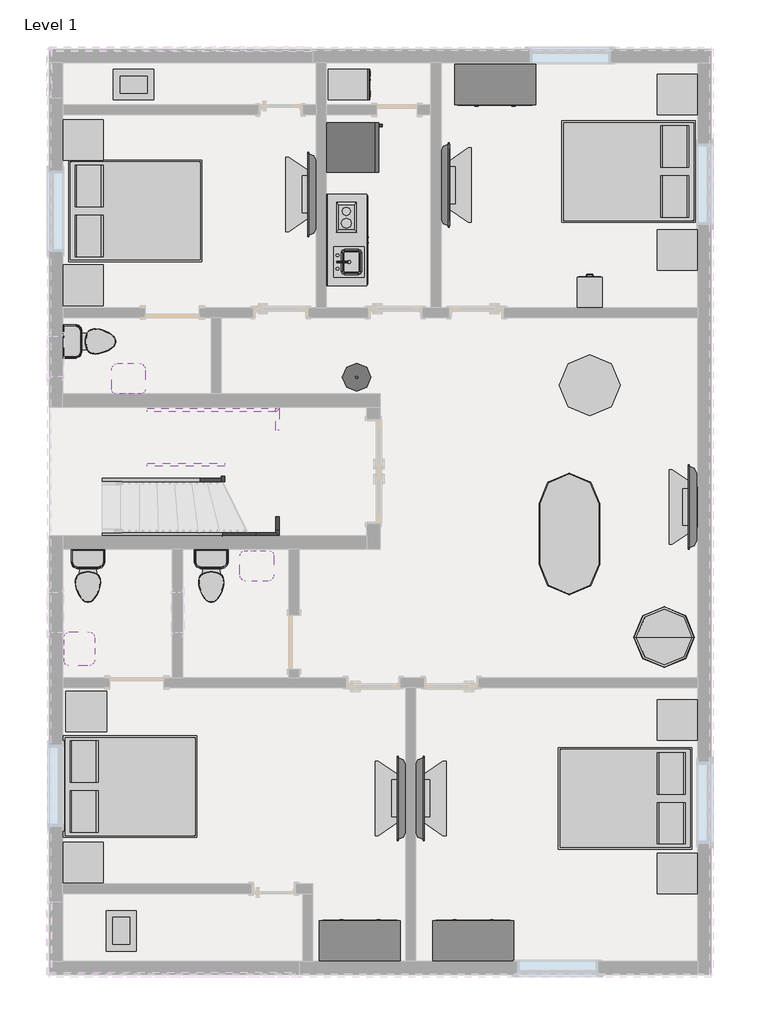
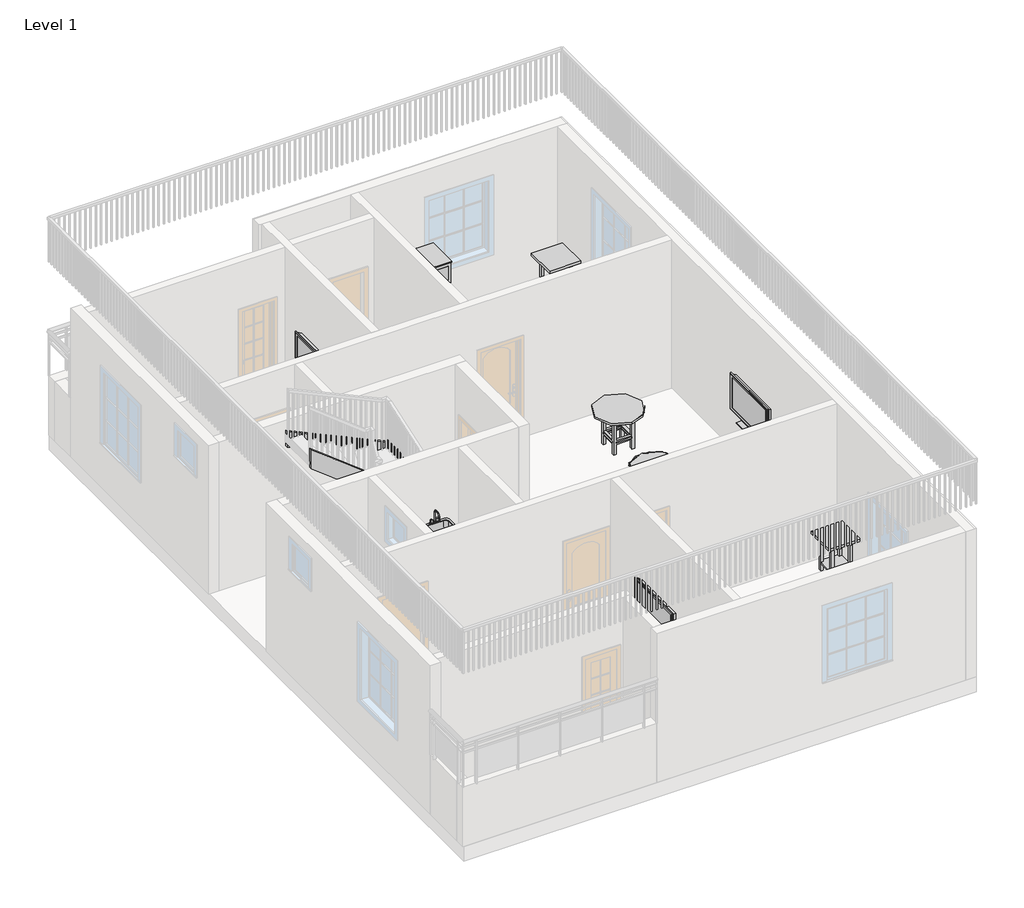
# One storey, part 7 of 7: 32 furniture elements, 10 members, 8 flow terminals, 4 proxies.
"""IFC4 building model written with IfcOpenShell, lengths in millimetres."""

from ifc_helpers import new_model, si_unit, frame, origin, place, context, project, spatial, polyline, outline, extrude, transform, mapped, element, save
from components import proxy_fe84b772, proxy_434a9211, proxy_844211aa, proxy_a13a33b2, flow_terminal_871c2e40, flow_terminal_d49f872f, flow_terminal_62a433f7, toilet_domestic_3d_toilet_domestic_3d_f7549cf7, toilet_domestic_3d_toilet_domestic_3d_183bbd19, furniture_1d2926bd, furniture_552c1472, furniture_95afb093, furniture_2babcf72, furniture_9fa109b2, furniture_fdf74506, tv_stand_tv_stand_6ce107e5, furniture_7122704d, furniture_2c34a4f9, furniture_905aceb5, furniture_5bc9ed15, furniture_c80d6d9c

model = new_model("IFC4")

# Units and contexts
model_context = context("Model", 3, world=origin())
ifc_project = project(units=[si_unit("LENGTHUNIT", "METRE", prefix="MILLI")], contexts=[model_context])

# Site, building, storey
site = spatial("IfcSite", under=ifc_project)
building = spatial("IfcBuilding", under=site)
storey = spatial("IfcBuildingStorey", under=building, Name="Level 1", Elevation=0.0)

# Proxies
placement = place(None, origin())
proxy_shape = proxy_fe84b772(model_context)
element("IfcBuildingElementProxy", 1, Name="Cook Top-2 Unit : 12\" x 18\"", ObjectType="Cook Top-2 Unit : 12\" x 18\"", at=placement, inside=storey, context=model_context, shape_type="MappedRepresentation", body=[
    mapped(proxy_shape, transform((-3933.68475, 9953.6087429, 0.0), x_axis=(-1.0, 0.0, 0.0), y_axis=(0.0, -1.0, 0.0), z_axis=(0.0, 0.0, 1.0))),
])
proxy_2_shape = proxy_434a9211(model_context)
element("IfcBuildingElementProxy", 2, Name="Dishwasher : 24\" x 24\" x 34\"", ObjectType="Dishwasher : 24\" x 24\" x 34\"", at=placement, inside=storey, context=model_context, shape_type="MappedRepresentation", body=[
    mapped(proxy_2_shape, transform((-3711.2966567, 11611.1664788, 0.0), x_axis=(0.0, 1.0, 0.0), y_axis=(-1.0, 0.0, 0.0), z_axis=(0.0, 0.0, 1.0))),
])
proxy_3_shape = proxy_844211aa(model_context)
element("IfcBuildingElementProxy", 3, Name="Kitchenette - Small : 54\"", ObjectType="Kitchenette - Small : 54\"", at=placement, inside=storey, context=model_context, shape_type="MappedRepresentation", body=[
    mapped(proxy_3_shape, transform((-4314.68475, 9561.7462424, 0.0), x_axis=(0.0, 1.0, 0.0), y_axis=(-1.0, 0.0, 0.0), z_axis=(0.0, 0.0, 1.0))),
])
proxy_4_shape = proxy_a13a33b2(model_context)
element("IfcBuildingElementProxy", 4, Name="Refrigerator.0001 : 30\" x 32\" RH", ObjectType="Refrigerator.0001 : 30\" x 32\" RH", at=placement, inside=storey, context=model_context, shape_type="MappedRepresentation", body=[
    mapped(proxy_4_shape, transform((-3941.62225, 10969.9349758, 0.0), x_axis=(0.0, 1.0000000000000002, 0.0), y_axis=(-1.0000000000000002, 0.0, 0.0), z_axis=(0.0, 0.0, 1.0))),
])

# Flow terminals
flow_terminal_shape = flow_terminal_871c2e40(model_context)
element("IfcFlowTerminal", 5, ObjectType="Sink Kitchen-Island : 18\" x 18\"", at=placement, inside=storey, context=model_context, shape_type="MappedRepresentation", body=[
    mapped(flow_terminal_shape, transform((-3969.4393489, 9234.5947068, 0.0), x_axis=(0.0, 1.0, 0.0), y_axis=(-1.0, 0.0, 0.0), z_axis=(0.0, 0.0, 1.0))),
])
flow_terminal_2_shape = flow_terminal_d49f872f(model_context)
element("IfcFlowTerminal", 6, ObjectType="Sink Vanity-Round : 19\" x 19\"", at=placement, inside=storey, context=model_context, shape_type="MappedRepresentation", body=[
    mapped(flow_terminal_2_shape, transform((-3760.8330095, 7600.5674621, 609.6), x_axis=(-1.0, 0.0, 0.0), y_axis=(0.0, -1.0, 0.0), z_axis=(0.0, 0.0, 1.0))),
])
flow_terminal_3_shape = flow_terminal_62a433f7(model_context)
element("IfcFlowTerminal", 7, ObjectType="Sink Vanity-Square : 20\" x 18\"", at=placement, inside=storey, context=model_context, shape_type="MappedRepresentation", body=[
    mapped(flow_terminal_3_shape, transform((-7270.7955095, 7449.2293485, 914.4), x_axis=(-1.0, 0.0, 0.0), y_axis=(0.0, -1.0, 0.0), z_axis=(0.0, 0.0, 1.0))),
])
element("IfcFlowTerminal", 8, ObjectType="Sink Vanity-Square : 20\" x 18\"", at=placement, inside=storey, context=model_context, shape_type="MappedRepresentation", body=[
    mapped(flow_terminal_3_shape, transform((-8071.5393489, 3417.9947068, 914.4), x_axis=(0.0, 1.0000000000000004, 0.0), y_axis=(-1.0000000000000004, 0.0, 0.0), z_axis=(0.0, 0.0, 1.0))),
])
element("IfcFlowTerminal", 9, ObjectType="Sink Vanity-Square : 20\" x 18\"", at=placement, inside=storey, context=model_context, shape_type="MappedRepresentation", body=[
    mapped(flow_terminal_3_shape, transform((-5371.7739906, 4726.7385462, 914.4), x_axis=(1.0, 0.0, 0.0), y_axis=(0.0, 1.0, 0.0), z_axis=(0.0, 0.0, 1.0))),
])
toilet_domestic_3d_toilet_domestic_3d_shape = toilet_domestic_3d_toilet_domestic_3d_f7549cf7(model_context)
toilet_domestic_3d_toilet_domestic_3d_2_shape = toilet_domestic_3d_toilet_domestic_3d_183bbd19(model_context)
element("IfcFlowTerminal", 10, ObjectType="Toilet-Domestic-3D : Toilet-Domestic-3D", at=placement, inside=storey, context=model_context, shape_type="MappedRepresentation", body=[
    mapped(toilet_domestic_3d_toilet_domestic_3d_shape, transform((-7896.08475, 4437.58792, 0.0), x_axis=(1.0, 0.0, 0.0), y_axis=(0.0, 1.0, 0.0), z_axis=(0.0, 0.0, 1.0))),
    mapped(toilet_domestic_3d_toilet_domestic_3d_2_shape, transform((-7896.08475, 4437.58792, 0.0), x_axis=(1.0, 0.0, 0.0), y_axis=(0.0, 1.0, 0.0), z_axis=(0.0, 0.0, 1.0))),
])
element("IfcFlowTerminal", 11, ObjectType="Toilet-Domestic-3D : Toilet-Domestic-3D", at=placement, inside=storey, context=model_context, shape_type="MappedRepresentation", body=[
    mapped(toilet_domestic_3d_toilet_domestic_3d_shape, transform((-6041.88475, 4437.58792, 0.0), x_axis=(1.0, 0.0, 0.0), y_axis=(0.0, 1.0, 0.0), z_axis=(0.0, 0.0, 1.0))),
    mapped(toilet_domestic_3d_toilet_domestic_3d_2_shape, transform((-6041.88475, 4437.58792, 0.0), x_axis=(1.0, 0.0, 0.0), y_axis=(0.0, 1.0, 0.0), z_axis=(0.0, 0.0, 1.0))),
])
element("IfcFlowTerminal", 12, ObjectType="Toilet-Domestic-3D : Toilet-Domestic-3D", at=placement, inside=storey, context=model_context, shape_type="MappedRepresentation", body=[
    mapped(toilet_domestic_3d_toilet_domestic_3d_shape, transform((-7782.3887227, 8056.4839473, 0.0), x_axis=(0.0, 1.0, 0.0), y_axis=(-1.0, 0.0, 0.0), z_axis=(0.0, 0.0, 1.0))),
    mapped(toilet_domestic_3d_toilet_domestic_3d_2_shape, transform((-7782.3887227, 8056.4839473, 0.0), x_axis=(0.0, 1.0, 0.0), y_axis=(-1.0, 0.0, 0.0), z_axis=(0.0, 0.0, 1.0))),
])

# Furniture
furniture_shape = furniture_1d2926bd(model_context)
element("IfcFurniture", 13, ObjectType="Bed-Box : Queen 60\" x 79\"", at=placement, inside=storey, context=model_context, shape_type="MappedRepresentation", body=[
    mapped(furniture_shape, transform((-7419.3142582, 9679.0364567, 0.0), x_axis=(0.0, 1.0, 0.0), y_axis=(-1.0, 0.0, 0.0), z_axis=(0.0, 0.0, 1.0))),
])
element("IfcFurniture", 14, ObjectType="Bed-Box : Queen 60\" x 79\"", at=placement, inside=storey, context=model_context, shape_type="MappedRepresentation", body=[
    mapped(furniture_shape, transform((466.3447582, 10948.3364064, 0.0), x_axis=(0.0, -1.0000000000000004, 0.0), y_axis=(1.0000000000000004, 0.0, 0.0), z_axis=(0.0, 0.0, 1.0))),
])
element("IfcFurniture", 15, ObjectType="Bed-Box : Queen 60\" x 79\"", at=placement, inside=storey, context=model_context, shape_type="MappedRepresentation", body=[
    mapped(furniture_shape, transform((-7495.5142582, 1024.4314883, 0.0), x_axis=(0.0, 1.0000000000000002, 0.0), y_axis=(-1.0000000000000002, 0.0, 0.0), z_axis=(0.0, 0.0, 1.0))),
])
element("IfcFurniture", 16, ObjectType="Bed-Box : Queen 60\" x 79\"", at=placement, inside=storey, context=model_context, shape_type="MappedRepresentation", body=[
    mapped(furniture_shape, transform((415.5447582, 1524.9364064, 0.0), x_axis=(0.0, -1.0000000000000002, 0.0), y_axis=(1.0000000000000002, 0.0, 0.0), z_axis=(0.0, 0.0, 1.0))),
])
furniture_2_shape = furniture_552c1472(model_context)
element("IfcFurniture", 17, ObjectType="Cabinet-File 3 Drawer : 15\" x 18\"", at=placement, inside=storey, context=model_context, shape_type="MappedRepresentation", body=[
    mapped(furniture_2_shape, transform((-480.1811971, 8650.9496472, 0.0), x_axis=(-1.0000000000000002, 0.0, 0.0), y_axis=(0.0, -1.0000000000000002, 0.0), z_axis=(0.0, 0.0, 1.0))),
])
furniture_3_shape = furniture_95afb093(model_context)
element("IfcFurniture", 18, ObjectType="Counter Top w Sink Hole : 24\" Depth", at=placement, inside=storey, context=model_context, shape_type="MappedRepresentation", body=[
    mapped(furniture_3_shape, transform((-4314.68475, 10095.1462424, 0.0), x_axis=(0.0, 1.0, 0.0), y_axis=(-1.0, 0.0, 0.0), z_axis=(0.0, 0.0, 1.0))),
])
furniture_4_shape = furniture_2babcf72(model_context)
element("IfcFurniture", 19, ObjectType="Dresser : 48\" x 60\" x 24\"", at=placement, inside=storey, context=model_context, shape_type="MappedRepresentation", body=[
    mapped(furniture_4_shape, transform((-1505.4914902, 12280.4469014, 0.0), x_axis=(1.0, 0.0, 0.0), y_axis=(0.0, 1.0, 0.0), z_axis=(0.0, 0.0, 1.0))),
])
furniture_5_shape = furniture_9fa109b2(model_context)
element("IfcFurniture", 20, ObjectType="Dresser : 48\" x 72\" x 24\"", at=placement, inside=storey, context=model_context, shape_type="MappedRepresentation", body=[
    mapped(furniture_5_shape, transform((-4075.8780099, -1323.6790068, 0.0), x_axis=(-1.0000000000000004, 0.0, 0.0), y_axis=(0.0, -1.0000000000000004, 0.0), z_axis=(0.0, 0.0, 1.0))),
])
element("IfcFurniture", 21, ObjectType="Dresser : 48\" x 72\" x 24\"", at=placement, inside=storey, context=model_context, shape_type="MappedRepresentation", body=[
    mapped(furniture_5_shape, transform((-2374.0780099, -1323.6790068, 0.0), x_axis=(-1.0000000000000004, 0.0, 0.0), y_axis=(0.0, -1.0000000000000004, 0.0), z_axis=(0.0, 0.0, 1.0))),
])
furniture_6_shape = furniture_fdf74506(model_context)
element("IfcFurniture", 22, ObjectType="TV - Flat Screen : 50\"", at=placement, inside=storey, context=model_context, shape_type="MappedRepresentation", body=[
    mapped(furniture_6_shape, transform((-2909.9461264, 1189.7284615, 914.4), x_axis=(0.0, 1.0000000000000002, 0.0), y_axis=(-1.0000000000000002, 0.0, 0.0), z_axis=(0.0, 0.0, 1.0))),
])
element("IfcFurniture", 23, ObjectType="TV - Flat Screen : 50\"", at=placement, inside=storey, context=model_context, shape_type="MappedRepresentation", body=[
    mapped(furniture_6_shape, transform((-4525.6233737, 10262.3394332, 914.4), x_axis=(0.0, -1.0, 0.0), y_axis=(1.0, 0.0, 0.0), z_axis=(0.0, 0.0, 1.0))),
])
element("IfcFurniture", 24, ObjectType="TV - Flat Screen : 50\"", at=placement, inside=storey, context=model_context, shape_type="MappedRepresentation", body=[
    mapped(furniture_6_shape, transform((-2528.9461264, 10409.9284615, 914.4), x_axis=(0.0, 1.0000000000000004, 0.0), y_axis=(-1.0000000000000004, 0.0, 0.0), z_axis=(0.0, 0.0, 1.0))),
])
element("IfcFurniture", 25, ObjectType="TV - Flat Screen : 50\"", at=placement, inside=storey, context=model_context, shape_type="MappedRepresentation", body=[
    mapped(furniture_6_shape, transform((-3179.4233737, 1181.8394332, 914.4), x_axis=(0.0, -1.0000000000000002, 0.0), y_axis=(1.0000000000000002, 0.0, 0.0), z_axis=(0.0, 0.0, 1.0))),
])
element("IfcFurniture", 26, ObjectType="TV - Flat Screen : 50\"", at=placement, inside=storey, context=model_context, shape_type="MappedRepresentation", body=[
    mapped(furniture_6_shape, transform((1196.1220775, 5563.3394332, 914.4), x_axis=(0.0, -1.0000000000000004, 0.0), y_axis=(1.0000000000000004, 0.0, 0.0), z_axis=(0.0, 0.0, 1.0))),
])
tv_stand_tv_stand_shape = tv_stand_tv_stand_6ce107e5(model_context)
element("IfcFurniture", 27, ObjectType="TV Stand : TV Stand", at=placement, inside=storey, context=model_context, shape_type="MappedRepresentation", body=[
    mapped(tv_stand_tv_stand_shape, transform((-4467.08475, 10391.4719494, 0.0), x_axis=(0.0, -1.0000000000000004, 0.0), y_axis=(1.0000000000000004, 0.0, 0.0), z_axis=(0.0, 0.0, 1.0))),
])
element("IfcFurniture", 28, ObjectType="TV Stand : TV Stand", at=placement, inside=storey, context=model_context, shape_type="MappedRepresentation", body=[
    mapped(tv_stand_tv_stand_shape, transform((-2587.48475, 10280.7959453, 0.0), x_axis=(0.0, 1.0000000000000002, 0.0), y_axis=(-1.0000000000000002, 0.0, 0.0), z_axis=(0.0, 0.0, 1.0))),
])
element("IfcFurniture", 29, ObjectType="TV Stand : TV Stand", at=placement, inside=storey, context=model_context, shape_type="MappedRepresentation", body=[
    mapped(tv_stand_tv_stand_shape, transform((-3120.88475, 1310.9719494, 0.0), x_axis=(0.0, -1.0000000000000002, 0.0), y_axis=(1.0000000000000002, 0.0, 0.0), z_axis=(0.0, 0.0, 1.0))),
])
element("IfcFurniture", 30, ObjectType="TV Stand : TV Stand", at=placement, inside=storey, context=model_context, shape_type="MappedRepresentation", body=[
    mapped(tv_stand_tv_stand_shape, transform((-2968.48475, 1060.5959453, 0.0), x_axis=(0.0, 1.0, 0.0), y_axis=(-1.0, 0.0, 0.0), z_axis=(0.0, 0.0, 1.0))),
])
element("IfcFurniture", 31, ObjectType="TV Stand : TV Stand", at=placement, inside=storey, context=model_context, shape_type="MappedRepresentation", body=[
    mapped(tv_stand_tv_stand_shape, transform((1298.71525, 5692.4719494, 0.0), x_axis=(0.0, -1.0, 0.0), y_axis=(1.0, 0.0, 0.0), z_axis=(0.0, 0.0, 1.0))),
])
furniture_7_shape = furniture_7122704d(model_context)
element("IfcFurniture", 32, ObjectType="Table-Coffee : 24\" x 24\" x 24\"", at=placement, inside=storey, context=model_context, shape_type="MappedRepresentation", body=[
    mapped(furniture_7_shape, transform((-7228.5505167, 11822.0728695, 0.0), x_axis=(1.0, 0.0, 0.0), y_axis=(0.0, 1.0, 0.0), z_axis=(0.0, 0.0, 1.0))),
])
element("IfcFurniture", 33, ObjectType="Table-Coffee : 24\" x 24\" x 24\"", at=placement, inside=storey, context=model_context, shape_type="MappedRepresentation", body=[
    mapped(furniture_7_shape, transform((-7300.2714016, -824.4514164, 0.0), x_axis=(0.0, 1.0000000000000002, 0.0), y_axis=(-1.0000000000000002, 0.0, 0.0), z_axis=(0.0, 0.0, 1.0))),
])
furniture_8_shape = furniture_2c34a4f9(model_context)
element("IfcFurniture", 34, ObjectType="Table-Dining Oval : 36\" x 72\"", at=placement, inside=storey, context=model_context, shape_type="MappedRepresentation", body=[
    mapped(furniture_8_shape, transform((-1015.1831107, 5562.7036195, 0.0), x_axis=(0.0, 1.0, 0.0), y_axis=(-1.0, 0.0, 0.0), z_axis=(0.0, 0.0, 1.0))),
])
furniture_9_shape = furniture_905aceb5(model_context)
element("IfcFurniture", 35, ObjectType="Table-Dining Round w Chairs : 36\" Diameter", at=placement, inside=storey, context=model_context, shape_type="MappedRepresentation", body=[
    mapped(furniture_9_shape, transform((-455.9667172, 7580.9626359, 0.0), x_axis=(1.0, 0.0, 0.0), y_axis=(0.0, 1.0, 0.0), z_axis=(0.0, 0.0, 1.0))),
])
furniture_10_shape = furniture_5bc9ed15(model_context)
element("IfcFurniture", 36, ObjectType="Table-Night Stand : 24\" x 24\" x 30\"", at=placement, inside=storey, context=model_context, shape_type="MappedRepresentation", body=[
    mapped(furniture_10_shape, transform((-8280.8183803, 8595.7889158, 0.0), x_axis=(1.0, 0.0, 0.0), y_axis=(0.0, 1.0, 0.0), z_axis=(0.0, 0.0, 1.0))),
])
element("IfcFurniture", 37, ObjectType="Table-Night Stand : 24\" x 24\" x 30\"", at=placement, inside=storey, context=model_context, shape_type="MappedRepresentation", body=[
    mapped(furniture_10_shape, transform((-8280.8183803, 10780.1889158, 0.0), x_axis=(1.0, 0.0, 0.0), y_axis=(0.0, 1.0, 0.0), z_axis=(0.0, 0.0, 1.0))),
])
element("IfcFurniture", 38, ObjectType="Table-Night Stand : 24\" x 24\" x 30\"", at=placement, inside=storey, context=model_context, shape_type="MappedRepresentation", body=[
    mapped(furniture_10_shape, transform((659.9816197, 11460.0839473, 0.0), x_axis=(1.0, 0.0, 0.0), y_axis=(0.0, 1.0, 0.0), z_axis=(0.0, 0.0, 1.0))),
])
element("IfcFurniture", 39, ObjectType="Table-Night Stand : 24\" x 24\" x 30\"", at=placement, inside=storey, context=model_context, shape_type="MappedRepresentation", body=[
    mapped(furniture_10_shape, transform((659.9816197, 9123.2839473, 0.0), x_axis=(1.0, 0.0, 0.0), y_axis=(0.0, 1.0, 0.0), z_axis=(0.0, 0.0, 1.0))),
])
element("IfcFurniture", 40, ObjectType="Table-Night Stand : 24\" x 24\" x 30\"", at=placement, inside=storey, context=model_context, shape_type="MappedRepresentation", body=[
    mapped(furniture_10_shape, transform((659.9816197, 2062.0839473, 0.0), x_axis=(1.0, 0.0, 0.0), y_axis=(0.0, 1.0, 0.0), z_axis=(0.0, 0.0, 1.0))),
])
element("IfcFurniture", 41, ObjectType="Table-Night Stand : 24\" x 24\" x 30\"", at=placement, inside=storey, context=model_context, shape_type="MappedRepresentation", body=[
    mapped(furniture_10_shape, transform((659.9816197, -249.3160527, 0.0), x_axis=(1.0, 0.0, 0.0), y_axis=(0.0, 1.0, 0.0), z_axis=(0.0, 0.0, 1.0))),
])
element("IfcFurniture", 42, ObjectType="Table-Night Stand : 24\" x 24\" x 30\"", at=placement, inside=storey, context=model_context, shape_type="MappedRepresentation", body=[
    mapped(furniture_10_shape, transform((-8280.8183803, -84.2160527, 0.0), x_axis=(1.0, 0.0, 0.0), y_axis=(0.0, 1.0, 0.0), z_axis=(0.0, 0.0, 1.0))),
])
element("IfcFurniture", 43, ObjectType="Table-Night Stand : 24\" x 24\" x 30\"", at=placement, inside=storey, context=model_context, shape_type="MappedRepresentation", body=[
    mapped(furniture_10_shape, transform((-8230.0183803, 2189.0839473, 0.0), x_axis=(1.0, 0.0, 0.0), y_axis=(0.0, 1.0, 0.0), z_axis=(0.0, 0.0, 1.0))),
])
furniture_11_shape = furniture_c80d6d9c(model_context)
element("IfcFurniture", 44, ObjectType="Table-Round : 36\" Diameter", at=placement, inside=storey, context=model_context, shape_type="MappedRepresentation", body=[
    mapped(furniture_11_shape, transform((765.31525, 3611.4839473, 0.0), x_axis=(1.0, 0.0, 0.0), y_axis=(0.0, 1.0, 0.0), z_axis=(0.0, 0.0, 1.0))),
])

# Members
element("IfcMember", 45, ObjectType="Stringer - 2\" Width", at=placement, inside=storey, context=model_context, shape_type="SweptSolid", body=[
    extrude(outline(polyline([(198.8692636, -7679.0298583), (0.0, -7679.0298583), (0.0, -7429.359774), (1046.1105277, -5889.48475), (1414.5925843, -5889.48475), (198.8692636, -7679.0298583)])), frame((0.0, 5948.2839473, 0.0), z_axis=(0.0, 1.0, 0.0), x_axis=(0.0, 0.0, 1.0)), (0.0, 0.0, 1.0), 50.8),
])
element("IfcMember", 46, ObjectType="Stringer - 2\" Width", at=placement, inside=storey, context=model_context, shape_type="SweptSolid", body=[
    extrude(outline(polyline([(5948.2839473, 1080.62139), (5948.2839473, 1699.1038993), (6149.5287831, 2074.4358445), (6176.8839473, 2074.4358445), (6176.8839473, 1480.4286626), (5962.5159726, 1080.62139), (5948.2839473, 1080.62139)])), frame((-5889.48475, 0.0, 0.0), z_axis=(1.0, 0.0, 0.0), x_axis=(0.0, 1.0, 0.0)), (0.0, 0.0, 1.0), 50.8),
])
element("IfcMember", 47, ObjectType="Stringer - 2\" Width", at=placement, inside=storey, context=model_context, shape_type="SweptSolid", body=[
    extrude(outline(polyline([(1686.9432948, -5838.68475), (2074.4358445, -5838.68475), (2990.3672313, -7005.4940547), (2602.8746816, -7005.4940547), (1686.9432948, -5838.68475)])), frame((0.0, 6176.8839473, 0.0), z_axis=(0.0, 1.0, 0.0), x_axis=(0.0, 0.0, 1.0)), (0.0, 0.0, 1.0), 50.8),
])
element("IfcMember", 48, ObjectType="Stringer - 2\" Width", at=placement, inside=storey, context=model_context, shape_type="SweptSolid", body=[
    extrude(outline(polyline([(224.2886171, -7679.0298583), (0.0, -7679.0298583), (0.0, -7453.2445978), (1129.7436444, -5370.1219368), (1476.4827863, -5370.1219368), (224.2886171, -7679.0298583)])), frame((0.0, 5128.1261204, 0.0), z_axis=(0.0, 1.0, 0.0), x_axis=(0.0, 0.0, 1.0)), (0.0, 0.0, 1.0), 50.8),
])
element("IfcMember", 49, ObjectType="Stringer - 2\" Width", at=placement, inside=storey, context=model_context, shape_type="SweptSolid", body=[
    extrude(outline(polyline([(-5370.1219368, 5128.1261204), (-5370.1219368, 5178.9261204), (-5069.3269231, 5178.9261204), (-5018.5269231, 5128.1261204), (-5370.1219368, 5128.1261204)])), frame((0.0, 0.0, 1129.7436444), z_axis=(0.0, 0.0, 1.0), x_axis=(1.0, 0.0, 0.0)), (0.0, 0.0, 1.0), 346.7391419),
])
element("IfcMember", 50, ObjectType="Stringer - 2\" Width", at=placement, inside=storey, context=model_context, shape_type="SweptSolid", body=[
    extrude(outline(polyline([(-5018.5269231, 5128.1261204), (-5069.3269231, 5178.9261204), (-5069.3269231, 5213.5040154), (-5018.5269231, 5213.5040154), (-5018.5269231, 5128.1261204)])), frame((0.0, 0.0, 1129.7436444), z_axis=(0.0, 0.0, 1.0), x_axis=(1.0, 0.0, 0.0)), (0.0, 0.0, 1.0), 346.7391419),
])
element("IfcMember", 51, ObjectType="Stringer - 2\" Width", at=placement, inside=storey, context=model_context, shape_type="SweptSolid", body=[
    extrude(outline(polyline([(5213.5040154, 1129.7436444), (5213.5040154, 1476.4827863), (6716.7832493, 1984.4827863), (6716.7832493, 1637.7436444), (5213.5040154, 1129.7436444)])), frame((-5069.3269231, 0.0, 0.0), z_axis=(1.0, 0.0, 0.0), x_axis=(0.0, 1.0, 0.0)), (0.0, 0.0, 1.0), 50.8),
])
element("IfcMember", 52, ObjectType="Stringer - 2\" Width", at=placement, inside=storey, context=model_context, shape_type="SweptSolid", body=[
    extrude(outline(polyline([(-5018.5269231, 6716.7832493), (-5069.3269231, 6716.7832493), (-5069.3269231, 6997.0417743), (-5018.5269231, 7047.8417743), (-5018.5269231, 6716.7832493)])), frame((0.0, 0.0, 1649.4430793), z_axis=(0.0, 0.0, 1.0), x_axis=(1.0, 0.0, 0.0)), (0.0, 0.0, 1.0), 321.7330066),
])
element("IfcMember", 53, ObjectType="Stringer - 2\" Width", at=placement, inside=storey, context=model_context, shape_type="SweptSolid", body=[
    extrude(outline(polyline([(-5018.5269231, 7047.8417743), (-5069.3269231, 6997.0417743), (-5079.1992765, 6997.0417743), (-5079.1992765, 7047.8417743), (-5018.5269231, 7047.8417743)])), frame((0.0, 0.0, 1649.4430793), z_axis=(0.0, 0.0, 1.0), x_axis=(1.0, 0.0, 0.0)), (0.0, 0.0, 1.0), 321.7330066),
])
element("IfcMember", 54, ObjectType="Stringer - 2\" Width", at=placement, inside=storey, context=model_context, shape_type="SweptSolid", body=[
    extrude(outline(polyline([(1649.4430793, -5079.1992765), (1971.176086, -5079.1992765), (2862.4513759, -7005.4940547), (2540.7183693, -7005.4940547), (1649.4430793, -5079.1992765)])), frame((0.0, 6997.0417743, 0.0), z_axis=(0.0, 1.0, 0.0), x_axis=(0.0, 0.0, 1.0)), (0.0, 0.0, 1.0), 50.8),
])

save(model, "model.ifc")

# Revit data of these elements
# Type "Cook Top-2 Unit : 12\" x 18\""
#   Assembly Code = "E1090400"
#   Counter Height = 3' - 0"
#   Depth = 1' - 6"
#   Width = 1' - 0"
#   Burner Material = Steel, Chrome Plated
#   Cooktop Material = Steel, Polished
#   Default Elevation = 0
# Type "Dishwasher : 24\" x 24\" x 34\""
#   Label = "DW"
#   Assembly Code = "E1090400"
#   Depth = 2' - 0"
#   Height = 2' - 10"
#   Width = 1' - 6"
#   Dishwasher Material = Steel, Paint Finish, Ivory, Glossy
#   Panel Face Material = Plastic, Opaque Black
#   Default Elevation = 0
# Type "Kitchenette - Small : 54\""
#   Assembly Code = "E1090400"
#   Width = 4' - 6"
#   Height = 2' - 10 1/2"
#   Depth = 2' - 0"
#   Toe Depth = 0' - 3"
#   Toe Height = 0' - 3 1/2"
#   Cabinet Material = Cabinets
#   Door/Drawer Material = Cabinets
#   Handle Material = Cabinets - Handles
#   Default Elevation = 0
# Type "Refrigerator.0001 : 30\" x 32\" RH"
#   Label = "REF."
#   Assembly Code = "E1090400"
#   Depth = 2' - 7 3/4"
#   Handle = 2' - 3"
#   Height = 5' - 10"
#   Rear Clearance = 0' - 2"
#   Top Door Height = 1' - 8"
#   Width = 2' - 5 3/8"
#   Material = Steel, Paint Finish, Ivory, Glossy
#   Default Elevation = 0
# Type "Sink Kitchen-Island : 18\" x 18\""
#   Assembly Code = "D2010410"
#   Counter Height = 3' - 0"
#   Depth = 1' - 6"
#   Width = 1' - 6"
#   Faucet Material = Steel, Polished
#   Sink Material = Steel, Polished
#   Default Elevation = 0
# Type "Sink Vanity-Round : 19\" x 19\""
#   Assembly Code = "D2010400"
#   Top Of Counter = 2' - 7"
#   Basin Material = Porcelain, Linen
#   Faucet Material = Steel, Polished
#   Default Elevation = 0
# Type "Sink Vanity-Square : 20\" x 18\""
#   Assembly Code = "D2010400"
#   Counter Height = 2' - 7"
#   Depth = 1' - 6"
#   Width = 1' - 8"
#   Basin Material = Porcelain, Linen
#   Faucet Material = Steel, Polished
#   Default Elevation = 0
# Type "Toilet-Domestic-3D : Toilet-Domestic-3D"
#   Assembly Code = "D2010110"
#   Toilet - Bowl/Basin Material = Porcelain, Linen
#   Toilet - Seat Material = Laminate, Linen, Matte
#   Default Elevation = 0
# Type "Bed-Box : Queen 60\" x 79\""
#   Assembly Code = "E2020200"
#   Length = 6' - 7"
#   Width = 5' - 0"
#   Frame Material = Birch
#   Mattress Material = Linen, White
#   Default Elevation = 0
# Type "Cabinet-File 3 Drawer : 15\" x 18\""
#   Assembly Code = "E2020200"
#   Depth = 1' - 6"
#   Height = 3' - 5"
#   Width = 1' - 3"
#   Cabinet Material = Steel, Paint Finish, Ivory, Glossy
#   Handle Material = Steel, Chrome Plated
#   Default Elevation = 0
# Type "Counter Top w Sink Hole : 24\" Depth"
#   Assembly Code = "C1030400"
#   Counter Thickness = 0' - 1 1/2"
#   Depth [instance default] = 2' - 1"
#   Height = 3' - 0"
#   Length [instance default] = 8' - 0"
#   Sink Location [instance default] = 2' - 0"
#   Sink Location To Wall [instance default] = 0' - 6"
#   Sink Opening Depth [instance default] = 1' - 3"
#   Sink Opening Width [instance default] = 2' - 3"
#   Counter Top Material = none
#   Default Elevation = 0
# Type "Dresser : 48\" x 60\" x 24\""
#   Assembly Code = "E2020200"
#   Depth = 2' - 0"
#   Height = 5' - 0"
#   Width = 4' - 0"
#   Dresser Material = Laminate - Ivory, Glossy
#   Drawer Material = Laminate, Ivory, Matte
#   Knob Material = Cherry
#   Default Elevation = 0
# Type "Dresser : 48\" x 72\" x 24\""
#   Assembly Code = "E2020200"
#   Depth = 2' - 0"
#   Height = 6' - 0"
#   Width = 4' - 0"
#   Dresser Material = Laminate - Ivory, Glossy
#   Drawer Material = Laminate, Ivory, Matte
#   Knob Material = Cherry
#   Default Elevation = 0
# Type "TV - Flat Screen : 50\""
#   SinAng = 0' - 0.0193"
#   L = 3' - 7.57782"
#   H = 2' - 0.51477"
#   Thickness = 0' - 4.33071"
#   Diagonal = 4' - 2"
#   CosAng = 0' - 0.03431"
#   Stand [instance default] = yes
#   Default Elevation = 0
# Type "TV Stand : TV Stand"
#   Depth = 1' - 6"
#   Width = 3' - 8"
#   Height = 1' - 7 1/2"
#   Finish = Melamine - Gray
#   Default Elevation = 0
# Type "Table-Coffee : 24\" x 24\" x 24\""
#   Assembly Code = "E2020200"
#   Height = 2' - 0"
#   Length = 2' - 0"
#   Width = 1' - 6"
#   Top Material = none
#   Frame Material = none
#   Default Elevation = 0
# Type "Table-Dining Oval : 36\" x 72\""
#   Assembly Code = "E2020200"
#   Length = 6' - 0"
#   Width = 3' - 0"
#   Base Material = Steel, Chrome Plated
#   Top Material = Glass - Clear, Grey
#   Default Elevation = 0
#   Description = (empty or 0)
# Type "Table-Dining Round w Chairs : 36\" Diameter"
#   Assembly Code = "E2020200"
#   Radius = 1' - 6"
#   Diameter = 3' - 0"
#   Height = 2' - 6"
#   Chairs = 4
#   Base Material = Pine
#   Top Material = Laminate, Linen, Matte
#   Default Elevation = 0
# Type "Table-Night Stand : 24\" x 24\" x 30\""
#   Assembly Code = "E2020200"
#   Depth = 2' - 0"
#   Height = 2' - 6"
#   Width = 2' - 0"
#   Base Material = Birch
#   Top Material = Laminate, Ivory, Matte
#   Default Elevation = 0
# Type "Table-Round : 36\" Diameter"
#   Assembly Code = "E2020200"
#   Base Radius = 0' - 10"
#   Height = 2' - 6"
#   Radius = 1' - 6"
#   Base Material = Steel, Chrome Plated
#   Top Material = Birch
#   Default Elevation = 0
# Element 1 (IfcBuildingElementProxy, "Cook Top-2 Unit : 12\" x 18\"")
#   Phase Created = New Construction
#   Materials on its faces: "Steel, Chrome Plated", "Steel, Polished"
# Element 2 (IfcBuildingElementProxy, "Dishwasher : 24\" x 24\" x 34\"")
#   Phase Created = New Construction
#   Materials on its faces: "Steel, Paint Finish, Ivory, Glossy", "Plastic, Opaque Black"
# Element 3 (IfcBuildingElementProxy, "Kitchenette - Small : 54\"")
#   Phase Created = New Construction
#   Materials on its faces: "Cabinets", "Cabinets - Handles"
# Element 4 (IfcBuildingElementProxy, "Refrigerator.0001 : 30\" x 32\" RH")
#   Phase Created = New Construction
#   Materials on its faces: "Steel, Paint Finish, Ivory, Glossy", "Steel, Chrome Plated"
# Element 5 (IfcFlowTerminal, "Sink Kitchen-Island : 18\" x 18\"")
#   Mark = "1"
#   Phase Created = New Construction
#   Materials on its faces: "Steel, Polished"
# Element 6 (IfcFlowTerminal, "Sink Vanity-Round : 19\" x 19\"")
#   Mark = "8"
#   Phase Created = New Construction
#   Materials on its faces: "Porcelain, Linen", "Steel, Polished"
# Element 7 (IfcFlowTerminal, "Sink Vanity-Square : 20\" x 18\"")
#   Mark = "5"
#   Phase Created = New Construction
#   Materials on its faces: "Porcelain, Linen", "Steel, Polished"
# Element 8 (IfcFlowTerminal, "Sink Vanity-Square : 20\" x 18\"")
#   Mark = "6"
#   Phase Created = New Construction
#   Materials on its faces: "Porcelain, Linen", "Steel, Polished"
# Element 9 (IfcFlowTerminal, "Sink Vanity-Square : 20\" x 18\"")
#   Mark = "7"
#   Phase Created = New Construction
#   Materials on its faces: "Porcelain, Linen", "Steel, Polished"
# Element 10 (IfcFlowTerminal, "Toilet-Domestic-3D : Toilet-Domestic-3D")
#   Mark = "2"
#   Phase Created = New Construction
#   Materials on its faces: "Porcelain, Linen", "Laminate, Linen, Matte"
# Element 11 (IfcFlowTerminal, "Toilet-Domestic-3D : Toilet-Domestic-3D")
#   Mark = "3"
#   Phase Created = New Construction
#   Materials on its faces: "Porcelain, Linen", "Laminate, Linen, Matte"
# Element 12 (IfcFlowTerminal, "Toilet-Domestic-3D : Toilet-Domestic-3D")
#   Mark = "4"
#   Phase Created = New Construction
#   Materials on its faces: "Porcelain, Linen", "Laminate, Linen, Matte"
# Elements 13, 14, 15, 16 (IfcFurniture, "Bed-Box : Queen 60\" x 79\"")
#   Phase Created = New Construction
#   Materials on its faces: "Birch", "Linen, White"
# Element 17 (IfcFurniture, "Cabinet-File 3 Drawer : 15\" x 18\"")
#   Phase Created = New Construction
#   Materials on its faces: "Steel, Chrome Plated", "Steel, Paint Finish, Ivory, Glossy"
# Element 18 (IfcFurniture, "Counter Top w Sink Hole : 24\" Depth")
#   Sink Opening Depth = 1' - 3"
#   Sink Location To Wall = 0' - 6"
#   Length = 4' - 6"
#   Sink Location = 1' - 2"
#   Sink Opening Width = 1' - 4"
#   Depth = 2' - 0"
#   Phase Created = New Construction
#   Materials on its faces: "Counter Top"
# Element 19 (IfcFurniture, "Dresser : 48\" x 60\" x 24\"")
#   Phase Created = New Construction
#   Materials on its faces: "Laminate, Ivory, Matte", "Cherry", "Laminate - Ivory, Glossy"
# Elements 20, 21 (IfcFurniture, "Dresser : 48\" x 72\" x 24\"")
#   Phase Created = New Construction
#   Materials on its faces: "Laminate, Ivory, Matte", "Cherry", "Laminate - Ivory, Glossy"
# Elements 22, 23, 24, 25, 26 (IfcFurniture, "TV - Flat Screen : 50\"")
#   Stand = yes
#   Phase Created = New Construction
#   Materials on its faces: "TV - Black", "TV - Glass", "TV - Screen"
# Elements 27, 28, 29, 30, 31 (IfcFurniture, "TV Stand : TV Stand")
#   Phase Created = New Construction
#   Materials on its faces: "Melamine - Gray", "Glass - Shelves"
# Elements 32, 33 (IfcFurniture, "Table-Coffee : 24\" x 24\" x 24\"")
#   Phase Created = New Construction
#   Materials on its faces: "Glass - Clear, Grey"
# Element 34 (IfcFurniture, "Table-Dining Oval : 36\" x 72\"")
#   Phase Created = New Construction
#   Materials on its faces: "Steel, Chrome Plated", "Glass - Clear, Grey"
# Element 35 (IfcFurniture, "Table-Dining Round w Chairs : 36\" Diameter")
#   Phase Created = New Construction
#   Materials on its faces: "Pine", "Laminate, Linen, Matte"
# Elements 36, 37, 38, 39, 40, 41, 42, 43 (IfcFurniture, "Table-Night Stand : 24\" x 24\" x 30\"")
#   Phase Created = New Construction
#   Materials on its faces: "Birch", "Laminate, Ivory, Matte"
# Element 44 (IfcFurniture, "Table-Round : 36\" Diameter")
#   Phase Created = New Construction
#   Materials on its faces: "Steel, Chrome Plated", "Birch"
# Elements 45, 46, 47, 48, 49, 50, 51, 52, 53, 54 (IfcMember, "Stringer - 2\" Width")
#   Phase Created = New Construction
# Materials
#   "Steel, Chrome Plated": class "Metal", colour RGB 17 17 17, transparency 0, Description = "Chromiuim plated steel", Cost = 0
#   "Steel, Polished": class "Metal", colour RGB 57 57 57, transparency 0, Description = "Polished steel", Cost = 0
#   "Steel, Paint Finish, Ivory, Glossy": class "Metal", colour RGB 247 247 239, transparency 0, Description = "Steel, paint finish, ivory, glossy", Cost = 0
#   "Plastic, Opaque Black": class "Plastic", colour RGB 0 0 0, transparency 0.7, Description = "Plastic, generic, opaque black", Cost = 0
#   "Cabinets": colour RGB 249 249 249, transparency 0
#   "Cabinets - Handles": class "Metal", colour RGB 57 57 57, transparency 0
#   "Porcelain, Linen": class "Ceramic", colour RGB 249 239 230, transparency 0, Description = "Porcelain, linen", Cost = 0
#   "Laminate, Linen, Matte": class "Plastic", colour RGB 249 239 230, transparency 0, Description = "Plastic Laminate - Linen, Matte", Cost = 0
#   "Birch": class "Wood", colour RGB 224 178 126, transparency 0, Description = "Betula Alleghaniensis", Cost = 0
#   "Linen, White": class "Textile", colour RGB 247 247 239, transparency 0, Description = "Linen, white", Cost = 0
#   "Laminate - Ivory, Glossy": colour RGB 247 247 239, transparency 0
#   "Laminate, Ivory, Matte": class "Plastic", colour RGB 247 247 239, transparency 0, Description = "Plastic Laminate - Ivory, Matte", Cost = 0
#   "Cherry": class "Wood", colour RGB 226 177 128, transparency 0, Description = "Prunus Serotina", Cost = 0
#   "Melamine - Gray": class "Wood", colour RGB 49 49 49, transparency 0
#   "Glass - Clear, Grey": class "Glass", colour RGB 252 255 255, transparency 0.64
#   "Pine": class "Wood", colour RGB 223 192 134, transparency 0, Description = "Pinus Echinata", Cost = 0
#   "Counter Top": class "Wood", colour RGB 226 177 128, transparency 0
#   "TV - Black": colour RGB 49 49 49, transparency 0
#   "TV - Glass": colour RGB 157 157 157, transparency 0.9
#   "TV - Screen": colour RGB 0 0 0, transparency 0
#   "Glass - Shelves": class "Glass", colour RGB 167 167 167, transparency 0.9
